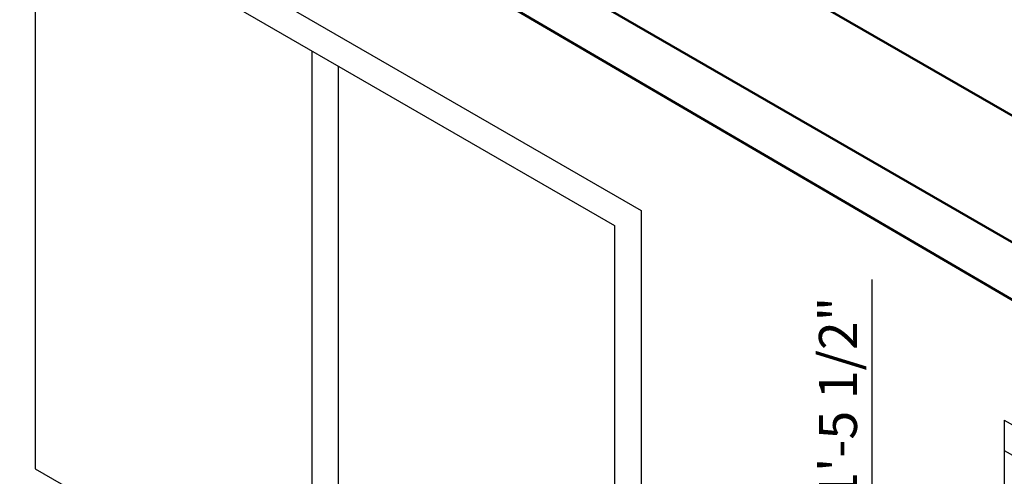
# Model space of a CAD drawing. Units: inches. Extents: x 5770 to 11891, y 3254 to 6808.
# Tile 12 of 15: x 6009 to 6073, y 3459 to 3489. Entities that reach past the tile are written whole.
import ezdxf

# ---------------------------------------------------------------- set-up
doc = ezdxf.new("R2010")
doc.units = ezdxf.units.IN
for name, color, linetype, lineweight in [('A-ANNO-DIMS', 2, 'Continuous', 18), ('A-DOOR', 4, 'Continuous', 25), ('A-FURN', 8, 'Continuous', 25), ('A-GLAZ', 4, 'Continuous', 25), ('A-WALL', 7, 'Continuous', 50)]:
    doc.layers.add(name, color=color, linetype=linetype, lineweight=lineweight)
doc.styles.get("Standard").update_dxf_attribs({"font": 'arial.ttf'})
doc.dimstyles.new('ISO-25', dxfattribs={"dimtxt": 2.5, "dimasz": 2.5, "dimexe": 1.25, "dimexo": 0.625, "dimtad": 1, "dimdec": 0, "dimlunit": 3, "dimtxsty": 'Standard', "dimcen": 2.5, "dimadec": 0, "dimazin": 0, "dimtfac": 1, "dimtdec": 0, "dimtmove": 0, "dimatfit": 3, "dimfxl": 1, "dimarcsym": 0})

# ---------------------------------------------------------------- blocks, each defined once
blk = doc.blocks.new('*D7')
at = {"layer": 'A-ANNO-DIMS', "color": 0, "lineweight": -2, "transparency": 16777216}
for p, q in [((5959.627, 3549.37), (5966.461, 3561.208)), ((5968.001, 3558.875), (6136.876, 3461.375)), ((6132.832, 3449.37), (6139.666, 3461.208))]:
    blk.add_line(p, q, dxfattribs=at)
at = {"layer": 'A-ANNO-DIMS', "color": 0, "transparency": 16777216}
for points in [[(5968.21, 3559.236), (5967.793, 3558.514), (5965.836, 3560.125)], [(6137.085, 3461.736), (6136.668, 3461.014), (6139.041, 3460.125)]]:
    blk.add_solid(points, dxfattribs=at)
at = {"layer": 'Defpoints', "color": 0, "transparency": 16777216}
for p in [(5959.314, 3548.829), (6139.041, 3460.125), (6132.519, 3448.829)]:
    blk.add_point(p, dxfattribs=at)
at = {"layer": 'A-ANNO-DIMS', "color": 0, "transparency": 16777216, "insert": (6061.618, 3507.021), "char_height": 2.5, "attachment_point": 5, "rotation": 330}
blk.add_mtext('16\'-8"', dxfattribs=at)
blk = doc.blocks.new('*D38')
at = {"layer": 'A-ANNO-DIMS', "color": 0, "lineweight": -2, "transparency": 16777216}
for p, q in [((6064.558, 3428.516), (6064.558, 3471.974)), ((6062.594, 3428.516), (6065.808, 3428.516)), ((6064.558, 3413.754), (6064.558, 3426.016)), ((6062.594, 3411.254), (6065.808, 3411.254))]:
    blk.add_line(p, q, dxfattribs=at)
at = {"layer": 'A-ANNO-DIMS', "color": 0, "transparency": 16777216}
for points in [[(6064.141, 3426.016), (6064.975, 3426.016), (6064.558, 3428.516)], [(6064.141, 3413.754), (6064.975, 3413.754), (6064.558, 3411.254)]]:
    blk.add_solid(points, dxfattribs=at)
at = {"layer": 'Defpoints', "color": 0, "transparency": 16777216}
for p in [(6061.969, 3428.516), (6064.558, 3428.516), (6061.969, 3411.254)]:
    blk.add_point(p, dxfattribs=at)
at = {"layer": 'A-ANNO-DIMS', "color": 0, "transparency": 16777216, "insert": (6062.64, 3451.495), "char_height": 2.5, "attachment_point": 5, "rotation": 90}
blk.add_mtext('POTTED PLANT 1\'-5 1/2"', dxfattribs=at)

msp = doc.modelspace()

# ---------------------------------------------------------------- linework, layer by layer
at = {"layer": 'A-DOOR'}
for p, q in [((6073.257, 3462.723), (6104.849, 3444.483)), ((6073.257, 3462.723), (6073.257, 3386.42)), ((6073.257, 3460.723), (6103.117, 3443.483))]:
    msp.add_line(p, q, dxfattribs=at)
at = {"layer": 'A-FURN'}
msp.add_line((6049.365, 3476.517), (6049.365, 3434.517), dxfattribs=at)
at = {"layer": 'A-GLAZ'}
for p, q in [((6007.795, 3500.517), (6049.365, 3476.517)), ((6009.528, 3497.517), (6047.633, 3475.517)), ((6009.528, 3497.517), (6009.528, 3459.517)), ((6027.714, 3487.017), (6027.714, 3449.017)), ((6029.446, 3486.017), (6029.446, 3448.017)), ((6047.633, 3475.517), (6047.633, 3437.517)), ((6009.528, 3459.517), (6047.633, 3437.517))]:
    msp.add_line(p, q, dxfattribs=at)
at = {"layer": 'A-WALL'}
for p, q in [((5959.314, 3548.829), (6132.519, 3448.829)), ((5959.314, 3540.508), (6115.241, 3450.483)), ((5974.02, 3529.017), (6111.683, 3448.429))]:
    msp.add_line(p, q, dxfattribs=at)

# ---------------------------------------------------------------- dimensions: what is measured, and where the dimension line sits
at = {"layer": 'A-ANNO-DIMS'}
dim = msp.add_linear_dim(base=(6139.041, 3460.125), p1=(5959.314, 3548.829), p2=(6132.519, 3448.829), angle=330, dimstyle='ISO-25', override={"dimclrd": 0, "dimclre": 0, "dimclrt": 0}, dxfattribs=at)
dim.commit()
dim.dimension.update_dxf_attribs({"geometry": '*D7', "text_midpoint": (6060.667, 3505.374), "dimtype": 161})
dim = msp.add_linear_dim(base=(6064.558, 3428.516), p1=(6061.969, 3411.254), p2=(6061.969, 3428.516), angle=90, text='POTTED PLANT <>', dimstyle='ISO-25', override={"dimdec": 1, "dimlfac": 1, "dimrnd": 0, "dimzin": 1, "dimdsep": 46, "dimlunit": 4, "dimfrac": 2}, dxfattribs=at)
dim.commit()
dim.dimension.update_dxf_attribs({"geometry": '*D38', "text_midpoint": (6062.64, 3451.495)})

doc.saveas('drawing.dxf')
